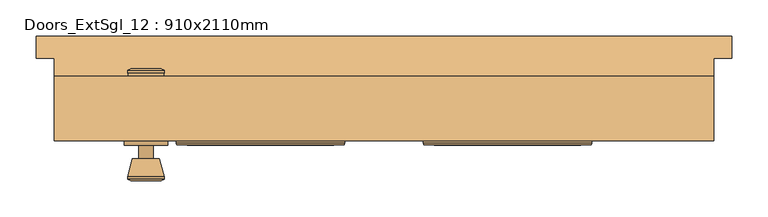
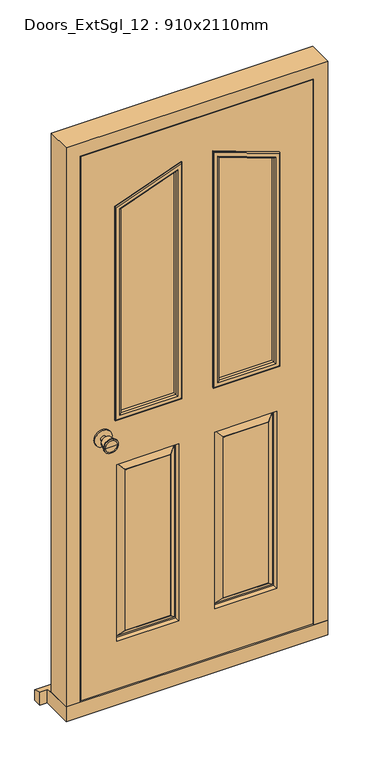
"""IFC4 building model written with IfcOpenShell, lengths in millimetres: door geometry, Doors_ExtSgl_12 : 910x2110mm."""

from ifc_helpers import new_model, si_unit, point, frame, frame_2d, origin, place, context, project, spatial, polyline, circle_curve, ellipse_curve, trimmed, segment, composite_curve, outline, extrude, faceted_brep, source, transform, mapped, element, save
from ifc_brep_helpers import plane_surface, cylinder_surface, revolved_surface, advanced_brep


def doors_extsgl_12_910x2110mm_9a09825e(model_context):
    return source(origin(), model_context, "Body", "SolidModel", [
        advanced_brep(
        [(-328.5, -18.4, 1000.0), (-318.5, -18.4, 1000.0), (-338.5, -18.4, 1000.0), (-308.0241324, -67.4, 1000.0), (-328.5, -67.4, 1000.0), (-348.9758676, -67.4, 1000.0), (-303.5, -65.5721319, 1000.0), (-353.5, -65.5721319, 1000.0), (-303.5, -62.1084537, 1000.0), (-353.5, -62.1084537, 1000.0), (-309.863764, -37.4, 1000.0), (-347.136236, -37.4, 1000.0), (-318.5, -37.4, 1000.0), (-338.5, -37.4, 1000.0)],
        [
            (0, 1),
            (1, 2, circle_curve(frame((-328.5, -18.4, 1000.0), z_axis=(0.0, 1.0, 0.0), x_axis=(-1.0, 0.0, 0.0)), 10.0)),
            (2, 0),
            (2, 1, circle_curve(frame((-328.5, -18.4, 1000.0), z_axis=(0.0, 1.0, 0.0), x_axis=(-1.0, 0.0, 0.0)), 10.0)),
            (3, 4),
            (4, 5),
            (5, 3, circle_curve(frame((-328.5, -67.4, 1000.0), z_axis=(0.0, -1.0, 0.0), x_axis=(-1.0, 0.0, 0.0)), 20.4758676)),
            (3, 5, circle_curve(frame((-328.5, -67.4, 1000.0), z_axis=(0.0, -1.0, 0.0), x_axis=(-1.0, 0.0, 0.0)), 20.4758676)),
            (6, 3),
            (5, 7),
            (7, 6, circle_curve(frame((-328.5, -65.5721319, 1000.0), z_axis=(0.0, -1.0, 0.0), x_axis=(-1.0, 0.0, 0.0)), 25.0)),
            (6, 7, circle_curve(frame((-328.5, -65.5721319, 1000.0), z_axis=(0.0, -1.0, 0.0), x_axis=(-1.0, 0.0, 0.0)), 25.0)),
            (8, 6),
            (7, 9),
            (9, 8, circle_curve(frame((-328.5, -62.1084537, 1000.0), z_axis=(0.0, -1.0, 0.0), x_axis=(-1.0, 0.0, 0.0)), 25.0)),
            (8, 9, circle_curve(frame((-328.5, -62.1084537, 1000.0), z_axis=(0.0, -1.0, 0.0), x_axis=(-1.0, 0.0, 0.0)), 25.0)),
            (10, 8),
            (9, 11),
            (11, 10, circle_curve(frame((-328.5, -37.4, 1000.0), z_axis=(0.0, -1.0, 0.0), x_axis=(-1.0, 0.0, 0.0)), 18.636236)),
            (10, 11, circle_curve(frame((-328.5, -37.4, 1000.0), z_axis=(0.0, -1.0, 0.0), x_axis=(-1.0, 0.0, 0.0)), 18.636236)),
            (12, 10),
            (11, 13),
            (13, 12, circle_curve(frame((-328.5, -37.4, 1000.0), z_axis=(0.0, -1.0, 0.0), x_axis=(-1.0, 0.0, 0.0)), 10.0)),
            (12, 13, circle_curve(frame((-328.5, -37.4, 1000.0), z_axis=(0.0, -1.0, 0.0), x_axis=(-1.0, 0.0, 0.0)), 10.0)),
            (1, 12),
            (13, 2),
        ],
        [
            plane_surface(frame((-328.5, -18.4, 1000.0), z_axis=(0.0, 1.0, 0.0), x_axis=(-1.0, 0.0, 0.0))),
            plane_surface(frame((-328.5, -67.4, 1000.0), z_axis=(0.0, -1.0, 0.0), x_axis=(-1.0, 0.0, 0.0))),
            revolved_surface(polyline([(-348.9758676, -67.4, 1000.0), (-353.5, -65.5721319, 1000.0)]), (-328.5, -18.4, 1000.0), (0.0, 1.0, 0.0)),
            cylinder_surface(frame((-328.5, -18.4, 1000.0), z_axis=(0.0, 1.0, 0.0), x_axis=(-1.0, 0.0, 0.0)), 25.0),
            revolved_surface(polyline([(-353.5, -62.1084537, 1000.0), (-347.136236, -37.4, 1000.0)]), (-328.5, -18.4, 1000.0), (0.0, 1.0, 0.0)),
            plane_surface(frame((-328.5, -37.4, 1000.0), z_axis=(0.0, 1.0, 0.0), x_axis=(-1.0, 0.0, 0.0))),
            cylinder_surface(frame((-328.5, -18.4, 1000.0), z_axis=(0.0, 1.0, 0.0), x_axis=(-1.0, 0.0, 0.0)), 10.0),
        ],
        [
            (0, [[1, 2, 3]]),
            (0, [[-3, 4, -1]]),
            (1, [[5, 6, 7]]),
            (1, [[-6, -5, 8]]),
            (2, [[9, -7, 10, 11]]),
            (2, [[-10, -8, -9, 12]]),
            (3, [[13, -11, 14, 15]]),
            (3, [[-14, -12, -13, 16]]),
            (4, [[17, -15, 18, 19]]),
            (4, [[-18, -16, -17, 20]]),
            (5, [[21, -19, 22, 23]]),
            (5, [[-22, -20, -21, 24]]),
            (6, [[25, -23, 26, -2]]),
            (6, [[-26, -24, -25, -4]]),
        ],
    ),
        extrude(outline(composite_curve([segment(trimmed(circle_curve(frame_2d((1000.0, -328.5)), 30.0), [point((1000.0, -358.5))], [point((1000.0, -298.5))], False, "CARTESIAN"), True, "CONTINUOUS"), segment(trimmed(circle_curve(frame_2d((1000.0, -328.5)), 30.0), [point((1000.0, -298.5))], [point((1000.0, -358.5))], False, "CARTESIAN"), True, "CONTINUOUS")], self_intersect=False)), frame((0.0, -18.4, 0.0), z_axis=(0.0, 1.0, 0.0), x_axis=(0.0, 0.0, 1.0)), (0.0, 0.0, 1.0), 6.0),
        advanced_brep(
        [(-328.5, 37.6, 1000.0), (-338.5, 37.6, 1000.0), (-318.5, 37.6, 1000.0), (-308.0241324, 86.6, 1000.0), (-348.9758676, 86.6, 1000.0), (-328.5, 86.6, 1000.0), (-303.5, 84.7721319, 1000.0), (-353.5, 84.7721319, 1000.0), (-303.5, 81.3084537, 1000.0), (-353.5, 81.3084537, 1000.0), (-309.863764, 56.6, 1000.0), (-347.136236, 56.6, 1000.0), (-318.5, 56.6, 1000.0), (-338.5, 56.6, 1000.0)],
        [
            (0, 1),
            (1, 2, circle_curve(frame((-328.5, 37.6, 1000.0), z_axis=(0.0, -1.0, 0.0), x_axis=(-1.0, 0.0, 0.0)), 10.0)),
            (2, 0),
            (2, 1, circle_curve(frame((-328.5, 37.6, 1000.0), z_axis=(0.0, -1.0, 0.0), x_axis=(-1.0, 0.0, 0.0)), 10.0)),
            (3, 4, circle_curve(frame((-328.5, 86.6, 1000.0), z_axis=(0.0, 1.0, 0.0), x_axis=(-1.0, 0.0, 0.0)), 20.4758676)),
            (4, 5),
            (5, 3),
            (4, 3, circle_curve(frame((-328.5, 86.6, 1000.0), z_axis=(0.0, 1.0, 0.0), x_axis=(-1.0, 0.0, 0.0)), 20.4758676)),
            (6, 7, circle_curve(frame((-328.5, 84.7721319, 1000.0), z_axis=(0.0, 1.0, 0.0), x_axis=(-1.0, 0.0, 0.0)), 25.0)),
            (7, 4),
            (3, 6),
            (7, 6, circle_curve(frame((-328.5, 84.7721319, 1000.0), z_axis=(0.0, 1.0, 0.0), x_axis=(-1.0, 0.0, 0.0)), 25.0)),
            (8, 9, circle_curve(frame((-328.5, 81.3084537, 1000.0), z_axis=(0.0, 1.0, 0.0), x_axis=(-1.0, 0.0, 0.0)), 25.0)),
            (9, 7),
            (6, 8),
            (9, 8, circle_curve(frame((-328.5, 81.3084537, 1000.0), z_axis=(0.0, 1.0, 0.0), x_axis=(-1.0, 0.0, 0.0)), 25.0)),
            (10, 11, circle_curve(frame((-328.5, 56.6, 1000.0), z_axis=(0.0, 1.0, 0.0), x_axis=(-1.0, 0.0, 0.0)), 18.636236)),
            (11, 9),
            (8, 10),
            (11, 10, circle_curve(frame((-328.5, 56.6, 1000.0), z_axis=(0.0, 1.0, 0.0), x_axis=(-1.0, 0.0, 0.0)), 18.636236)),
            (12, 13, circle_curve(frame((-328.5, 56.6, 1000.0), z_axis=(0.0, 1.0, 0.0), x_axis=(-1.0, 0.0, 0.0)), 10.0)),
            (13, 11),
            (10, 12),
            (13, 12, circle_curve(frame((-328.5, 56.6, 1000.0), z_axis=(0.0, 1.0, 0.0), x_axis=(-1.0, 0.0, 0.0)), 10.0)),
            (1, 13),
            (12, 2),
        ],
        [
            plane_surface(frame((-328.5, 37.6, 1000.0), z_axis=(0.0, -1.0, 0.0), x_axis=(-1.0, 0.0, 0.0))),
            plane_surface(frame((-328.5, 86.6, 1000.0), z_axis=(0.0, 1.0, 0.0), x_axis=(-1.0, 0.0, 0.0))),
            revolved_surface(polyline([(-348.9758676, 86.6, 1000.0), (-353.5, 84.7721319, 1000.0)]), (-328.5, 37.6, 1000.0), (0.0, -1.0, 0.0)),
            cylinder_surface(frame((-328.5, 37.6, 1000.0), z_axis=(0.0, -1.0, 0.0), x_axis=(-1.0, 0.0, 0.0)), 25.0),
            revolved_surface(polyline([(-353.5, 81.3084537, 1000.0), (-347.136236, 56.6, 1000.0)]), (-328.5, 37.6, 1000.0), (0.0, -1.0, 0.0)),
            plane_surface(frame((-328.5, 56.6, 1000.0), z_axis=(0.0, -1.0, 0.0), x_axis=(-1.0, 0.0, 0.0))),
            cylinder_surface(frame((-328.5, 37.6, 1000.0), z_axis=(0.0, -1.0, 0.0), x_axis=(-1.0, 0.0, 0.0)), 10.0),
        ],
        [
            (0, [[1, 2, 3]]),
            (0, [[-3, 4, -1]]),
            (1, [[5, 6, 7]]),
            (1, [[8, -7, -6]]),
            (2, [[9, 10, -5, 11]]),
            (2, [[12, -11, -8, -10]]),
            (3, [[13, 14, -9, 15]]),
            (3, [[16, -15, -12, -14]]),
            (4, [[17, 18, -13, 19]]),
            (4, [[20, -19, -16, -18]]),
            (5, [[21, 22, -17, 23]]),
            (5, [[24, -23, -20, -22]]),
            (6, [[-2, 25, -21, 26]]),
            (6, [[-4, -26, -24, -25]]),
        ],
    ),
        extrude(outline(composite_curve([segment(trimmed(circle_curve(frame_2d((1000.0, -328.5)), 30.0), [point((1000.0, -358.5))], [point((1000.0, -298.5))], False, "CARTESIAN"), True, "CONTINUOUS"), segment(trimmed(circle_curve(frame_2d((1000.0, -328.5)), 30.0), [point((1000.0, -298.5))], [point((1000.0, -358.5))], False, "CARTESIAN"), True, "CONTINUOUS")], self_intersect=False)), frame((0.0, 31.6, 0.0), z_axis=(0.0, 1.0, 0.0), x_axis=(0.0, 0.0, 1.0)), (0.0, 0.0, 1.0), 6.0),
        faceted_brep([(384.5, 76.6, 54.5), (455.0, 76.6, 54.5), (455.0, -12.4, 54.5), (406.5, -12.4, 54.5), (406.5, 34.6, 54.5), (384.5, 34.6, 54.5), (384.5, 76.6, 2039.5), (-384.5, 76.6, 2039.5), (-384.5, 76.6, 54.5), (-455.0, 76.6, 54.5), (-455.0, 76.6, 2110.0), (455.0, 76.6, 2110.0), (455.0, -12.4, 2110.0), (-455.0, -12.4, 2110.0), (-455.0, -12.4, 54.5), (-406.5, -12.4, 54.5), (-406.5, -12.4, 2061.5), (406.5, -12.4, 2061.5), (406.5, 34.6, 2061.5), (-406.5, 34.6, 2061.5), (-406.5, 34.6, 54.5), (-384.5, 34.6, 54.5), (-384.5, 34.6, 2039.5), (384.5, 34.6, 2039.5)], [[[0, 1, 2, 3, 4, 5]], [[1, 0, 6, 7, 8, 9, 10, 11]], [[2, 1, 11, 12]], [[3, 2, 12, 13, 14, 15, 16, 17]], [[4, 3, 17, 18]], [[5, 4, 18, 19, 20, 21, 22, 23]], [[0, 5, 23, 6]], [[8, 7, 22, 21]], [[9, 8, 21, 20, 15, 14]], [[10, 9, 14, 13]], [[16, 15, 20, 19]], [[11, 10, 13, 12]], [[17, 16, 19, 18]], [[7, 6, 23, 22]]]),
        faceted_brep([(403.5, -12.4, 58.5), (403.5, -12.4, 2058.5), (-404.4250294, -12.4, 2058.5), (-404.4250294, -12.4, 58.5), (62.5, -12.4, 1058.5), (62.5, -12.4, 1908.5), (278.5, -12.4, 1829.8824294), (278.5, -12.4, 1058.5), (-278.5, -12.4, 1058.5), (-278.5, -12.4, 1829.8824294), (-62.5, -12.4, 1908.5), (-62.5, -12.4, 1058.5), (-62.5, -12.4, 883.5), (-62.5, -12.4, 233.5), (-278.5, -12.4, 233.5), (-278.5, -12.4, 883.5), (278.5, -12.4, 883.5), (278.5, -12.4, 233.5), (62.5, -12.4, 233.5), (62.5, -12.4, 883.5), (-92.5, -12.4, 263.5), (-92.5, -12.4, 853.5), (-248.5, -12.4, 853.5), (-248.5, -12.4, 263.5), (248.5, -12.4, 263.5), (248.5, -12.4, 853.5), (92.5, -12.4, 853.5), (92.5, -12.4, 263.5), (403.5, 31.6, 58.5), (-404.4250294, 31.6, 58.5), (-404.4250294, 31.6, 2058.5), (403.5, 31.6, 2058.5), (62.5, 31.6, 1058.5), (278.5, 31.6, 1058.5), (278.5, 31.6, 1829.8824294), (62.5, 31.6, 1908.5), (-278.5, 31.6, 1058.5), (-62.5, 31.6, 1058.5), (-62.5, 31.6, 1908.5), (-278.5, 31.6, 1829.8824294), (62.5, 31.6, 883.5), (62.5, 31.6, 233.5), (278.5, 31.6, 233.5), (278.5, 31.6, 883.5), (-278.5, 31.6, 883.5), (-278.5, 31.6, 233.5), (-62.5, 31.6, 233.5), (-62.5, 31.6, 883.5), (92.5, 31.6, 263.5), (92.5, 31.6, 853.5), (248.5, 31.6, 853.5), (248.5, 31.6, 263.5), (-248.5, 31.6, 263.5), (-248.5, 31.6, 853.5), (-92.5, 31.6, 853.5), (-92.5, 31.6, 263.5), (65.5, 16.6, 880.5), (65.5, 16.6, 236.5), (90.5, 30.6, 855.5), (90.5, 30.6, 261.5), (70.5, 16.6, 241.5), (70.5, 16.6, 875.5), (92.5, 30.6, 263.5), (92.5, 30.6, 853.5), (275.5, 16.6, 236.5), (250.5, 30.6, 261.5), (270.5, 16.6, 241.5), (248.5, 30.6, 263.5), (275.5, 16.6, 880.5), (250.5, 30.6, 855.5), (270.5, 16.6, 875.5), (248.5, 30.6, 853.5), (-275.5, 16.6, 880.5), (-275.5, 16.6, 236.5), (-250.5, 30.6, 855.5), (-250.5, 30.6, 261.5), (-270.5, 16.6, 241.5), (-270.5, 16.6, 875.5), (-248.5, 30.6, 263.5), (-248.5, 30.6, 853.5), (-65.5, 16.6, 236.5), (-90.5, 30.6, 261.5), (-70.5, 16.6, 241.5), (-92.5, 30.6, 263.5), (-65.5, 16.6, 880.5), (-90.5, 30.6, 855.5), (-70.5, 16.6, 875.5), (-92.5, 30.6, 853.5), (-92.5, -11.4, 263.5), (-92.5, -11.4, 853.5), (-70.5, 2.6, 241.5), (-70.5, 2.6, 875.5), (-90.5, -11.4, 855.5), (-90.5, -11.4, 261.5), (-65.5, 2.6, 880.5), (-65.5, 2.6, 236.5), (-248.5, -11.4, 853.5), (-270.5, 2.6, 875.5), (-250.5, -11.4, 855.5), (-275.5, 2.6, 880.5), (-248.5, -11.4, 263.5), (-270.5, 2.6, 241.5), (-250.5, -11.4, 261.5), (-275.5, 2.6, 236.5), (275.5, 2.6, 880.5), (275.5, 2.6, 236.5), (250.5, -11.4, 855.5), (250.5, -11.4, 261.5), (270.5, 2.6, 241.5), (270.5, 2.6, 875.5), (248.5, -11.4, 263.5), (248.5, -11.4, 853.5), (65.5, 2.6, 236.5), (90.5, -11.4, 261.5), (70.5, 2.6, 241.5), (92.5, -11.4, 263.5), (65.5, 2.6, 880.5), (90.5, -11.4, 855.5), (70.5, 2.6, 875.5), (92.5, -11.4, 853.5)], [[[0, 1, 2, 3], [4, 5, 6, 7], [8, 9, 10, 11], [12, 13, 14, 15], [16, 17, 18, 19]], [[20, 21, 22, 23]], [[24, 25, 26, 27]], [[28, 29, 30, 31], [32, 33, 34, 35], [36, 37, 38, 39], [40, 41, 42, 43], [44, 45, 46, 47]], [[48, 49, 50, 51]], [[52, 53, 54, 55]], [[1, 0, 28, 31]], [[2, 1, 31, 30]], [[3, 2, 30, 29]], [[0, 3, 29, 28]], [[5, 4, 32, 35]], [[6, 5, 35, 34]], [[7, 6, 34, 33]], [[4, 7, 33, 32]], [[9, 8, 36, 39]], [[10, 9, 39, 38]], [[11, 10, 38, 37]], [[8, 11, 37, 36]], [[56, 57, 41, 40]], [[58, 59, 60, 61]], [[48, 62, 63, 49]], [[41, 57, 64, 42]], [[60, 59, 65, 66]], [[62, 48, 51, 67]], [[42, 64, 68, 43]], [[66, 65, 69, 70]], [[67, 51, 50, 71]], [[56, 40, 43, 68]], [[57, 56, 68, 64], [61, 60, 66, 70]], [[58, 61, 70, 69]], [[59, 58, 69, 65], [63, 62, 67, 71]], [[49, 63, 71, 50]], [[72, 73, 45, 44]], [[74, 75, 76, 77]], [[52, 78, 79, 53]], [[45, 73, 80, 46]], [[76, 75, 81, 82]], [[78, 52, 55, 83]], [[46, 80, 84, 47]], [[82, 81, 85, 86]], [[83, 55, 54, 87]], [[72, 44, 47, 84]], [[73, 72, 84, 80], [77, 76, 82, 86]], [[74, 77, 86, 85]], [[75, 74, 85, 81], [79, 78, 83, 87]], [[53, 79, 87, 54]], [[88, 89, 21, 20]], [[90, 91, 92, 93]], [[12, 94, 95, 13]], [[21, 89, 96, 22]], [[92, 91, 97, 98]], [[94, 12, 15, 99]], [[22, 96, 100, 23]], [[98, 97, 101, 102]], [[99, 15, 14, 103]], [[88, 20, 23, 100]], [[93, 92, 98, 102], [89, 88, 100, 96]], [[90, 93, 102, 101]], [[95, 94, 99, 103], [91, 90, 101, 97]], [[13, 95, 103, 14]], [[104, 105, 17, 16]], [[106, 107, 108, 109]], [[24, 110, 111, 25]], [[17, 105, 112, 18]], [[108, 107, 113, 114]], [[110, 24, 27, 115]], [[18, 112, 116, 19]], [[114, 113, 117, 118]], [[115, 27, 26, 119]], [[104, 16, 19, 116]], [[105, 104, 116, 112], [109, 108, 114, 118]], [[106, 109, 118, 117]], [[107, 106, 117, 113], [111, 110, 115, 119]], [[25, 111, 119, 26]]]),
        faceted_brep([(480.0, 131.6, 0.0), (480.0, 131.6, 38.5947221), (480.0, 101.6, 47.2703282), (480.0, 101.6, 0.0), (-480.0, 131.6, 38.5947221), (-480.0, 131.6, 0.0), (-480.0, 101.6, 0.0), (-480.0, 101.6, 47.2703282), (455.0, 101.6, 0.0), (455.0, -12.4, 0.0), (-455.0, -12.4, 0.0), (-455.0, 101.6, 0.0), (-455.0, 101.6, 47.2703282), (-455.0, 76.6, 54.5), (455.0, 76.6, 54.5), (455.0, 101.6, 47.2703282), (-455.0, -12.4, 54.5), (455.0, -12.4, 54.5)], [[[0, 1, 2, 3]], [[4, 5, 6, 7]], [[5, 0, 3, 8, 9, 10, 11, 6]], [[1, 0, 5, 4]], [[1, 4, 7, 12, 13, 14, 15, 2]], [[13, 16, 17, 14]], [[16, 10, 9, 17]], [[12, 11, 10, 16, 13]], [[11, 12, 7, 6]], [[8, 15, 14, 17, 9]], [[15, 8, 3, 2]]]),
        extrude(outline(polyline([(1058.5, 278.5), (1829.8824294, 278.5), (1908.5, 62.5), (1058.5, 62.5), (1058.5, 278.5)])), frame((0.0, -2.4, 0.0), z_axis=(0.0, 1.0, 0.0), x_axis=(0.0, 0.0, 1.0)), (0.0, 0.0, 1.0), 24.0),
        extrude(outline(polyline([(1058.5, -62.5), (1908.5, -62.5), (1829.8824294, -278.5), (1058.5, -278.5), (1058.5, -62.5)])), frame((0.0, -2.4, 0.0), z_axis=(0.0, 1.0, 0.0), x_axis=(0.0, 0.0, 1.0)), (0.0, 0.0, 1.0), 24.0),
        advanced_brep(
        [(286.5, 35.6, 1835.4840897), (286.5, 31.6, 1835.4840897), (286.5, 31.6, 1050.5), (286.5, 35.6, 1050.5), (284.5, 37.6, 1834.0836746), (284.5, 37.6, 1052.5), (266.5, 32.6, 1821.4799389), (271.5, 37.6, 1824.9809766), (271.5, 37.6, 1065.5), (266.5, 32.6, 1070.5), (266.5, 21.6, 1821.4799389), (266.5, 21.6, 1070.5), (278.5, 31.6, 1829.8824294), (278.5, 21.6, 1829.8824294), (278.5, 21.6, 1058.5), (278.5, 31.6, 1058.5), (54.5, 31.6, 1050.5), (54.5, 35.6, 1050.5), (56.5, 37.6, 1052.5), (69.5, 37.6, 1065.5), (74.5, 32.6, 1070.5), (74.5, 21.6, 1070.5), (62.5, 21.6, 1058.5), (62.5, 31.6, 1058.5), (54.5, 31.6, 1919.9251841), (54.5, 35.6, 1919.9251841), (56.5, 37.6, 1917.068888), (69.5, 37.6, 1898.502964), (74.5, 32.6, 1891.3622239), (74.5, 21.6, 1891.3622239), (62.5, 21.6, 1908.5), (62.5, 31.6, 1908.5)],
        [
            (0, 1),
            (1, 2),
            (2, 3),
            (3, 0),
            (4, 0, ellipse_curve(frame((284.5, 35.6, 1834.0836746), z_axis=(0.5735764363510463, 0.0, -0.8191520442889918), x_axis=(0.8191520442889918, 0.0, 0.5735764363510459)), 2.4415492, 2.0)),
            (3, 5, ellipse_curve(frame((284.5, 35.6, 1052.5), z_axis=(0.7071067811865475, 0.0, 0.7071067811865475), x_axis=(-0.7071067811865474, 0.0, 0.7071067811865476)), 2.8284271, 2.0)),
            (5, 4),
            (6, 7, ellipse_curve(frame((271.5, 32.6, 1824.9809766), z_axis=(0.5735764363510463, 0.0, -0.8191520442889918), x_axis=(0.8191520442889918, 0.0, 0.5735764363510459)), 6.1038729, 5.0)),
            (7, 8),
            (8, 9, ellipse_curve(frame((271.5, 32.6, 1065.5), z_axis=(0.7071067811865475, 0.0, 0.7071067811865475), x_axis=(-0.7071067811865474, 0.0, 0.7071067811865476)), 7.0710678, 5.0)),
            (9, 6),
            (10, 6),
            (9, 11),
            (11, 10),
            (12, 13),
            (13, 14),
            (14, 15),
            (15, 12),
            (2, 16),
            (16, 17),
            (17, 3),
            (17, 18, ellipse_curve(frame((56.5, 35.6, 1052.5), z_axis=(0.7071067811865475, 0.0, -0.7071067811865475), x_axis=(0.7071067811865476, 0.0, 0.7071067811865474)), 2.8284271, 2.0)),
            (18, 5),
            (8, 19),
            (19, 20, ellipse_curve(frame((69.5, 32.6, 1065.5), z_axis=(0.7071067811865475, 0.0, -0.7071067811865475), x_axis=(0.7071067811865476, 0.0, 0.7071067811865474)), 7.0710678, 5.0)),
            (20, 9),
            (20, 21),
            (21, 11),
            (14, 22),
            (22, 23),
            (23, 15),
            (16, 24),
            (24, 25),
            (25, 17),
            (25, 26, ellipse_curve(frame((56.5, 35.6, 1917.068888), z_axis=(-0.8191520442889917, 0.0, -0.5735764363510462), x_axis=(0.5735764363510462, 0.0, -0.8191520442889918)), 3.4868936, 2.0)),
            (26, 18),
            (19, 27),
            (27, 28, ellipse_curve(frame((69.5, 32.6, 1898.502964), z_axis=(-0.8191520442889917, 0.0, -0.5735764363510462), x_axis=(0.5735764363510462, 0.0, -0.8191520442889918)), 8.717234, 5.0)),
            (28, 20),
            (28, 29),
            (29, 21),
            (22, 30),
            (30, 31),
            (31, 23),
            (24, 1),
            (0, 25),
            (4, 26),
            (7, 27),
            (6, 28),
            (10, 29),
            (13, 30),
            (12, 31),
        ],
        [
            plane_surface(frame((286.5, 31.6, 1835.4840897), z_axis=(1.0, 0.0, 0.0), x_axis=(0.0, 0.0, -1.0))),
            cylinder_surface(frame((284.5, 35.6, 1829.8824294), z_axis=(0.0, 0.0, 1.0), x_axis=(1.0, 0.0, 0.0)), 2.0),
            cylinder_surface(frame((271.5, 32.6, 1829.8824294), z_axis=(0.0, 0.0, 1.0), x_axis=(1.0, 0.0, 0.0)), 5.0),
            plane_surface(frame((266.5, 32.6, 1821.4799389), z_axis=(-1.0, 0.0, 0.0), x_axis=(0.0, 0.0, -1.0))),
            plane_surface(frame((278.5, 21.6, 1829.8824294), z_axis=(1.0, 0.0, 0.0), x_axis=(0.0, 0.0, -1.0))),
            plane_surface(frame((286.5, 31.6, 1050.5), z_axis=(0.0, 0.0, -1.0), x_axis=(-1.0, 0.0, 0.0))),
            cylinder_surface(frame((278.5, 35.6, 1052.5), z_axis=(1.0, 0.0, 0.0), x_axis=(0.0, 0.0, -1.0)), 2.0),
            cylinder_surface(frame((278.5, 32.6, 1065.5), z_axis=(1.0, 0.0, 0.0), x_axis=(0.0, 0.0, -1.0)), 5.0),
            plane_surface(frame((266.5, 32.6, 1070.5), z_axis=(0.0, 0.0, 1.0), x_axis=(-1.0, 0.0, 0.0))),
            plane_surface(frame((278.5, 21.6, 1058.5), z_axis=(0.0, 0.0, -1.0), x_axis=(-1.0, 0.0, 0.0))),
            plane_surface(frame((54.5, 31.6, 1050.5), z_axis=(-1.0, 0.0, 0.0), x_axis=(0.0, 0.0, 1.0))),
            cylinder_surface(frame((56.5, 35.6, 1058.5), z_axis=(0.0, 0.0, -1.0), x_axis=(-1.0, 0.0, 0.0)), 2.0),
            cylinder_surface(frame((69.5, 32.6, 1058.5), z_axis=(0.0, 0.0, -1.0), x_axis=(-1.0, 0.0, 0.0)), 5.0),
            plane_surface(frame((74.5, 32.6, 1070.5), z_axis=(1.0, 0.0, 0.0), x_axis=(0.0, 0.0, 1.0))),
            plane_surface(frame((62.5, 21.6, 1058.5), z_axis=(-1.0, 0.0, 0.0), x_axis=(0.0, 0.0, 1.0))),
            plane_surface(frame((54.5, 31.6, 1919.9251841), z_axis=(0.3420201433256683, 0.0, 0.9396926207859085), x_axis=(0.9396926207859085, 0.0, -0.3420201433256683))),
            cylinder_surface(frame((64.5521209, 35.6, 1914.1381557), z_axis=(-0.9396926207859085, 0.0, 0.34202014332566844), x_axis=(0.34202014332566844, 0.0, 0.9396926207859085)), 2.0),
            plane_surface(frame((56.5, 37.6, 1917.068888), z_axis=(0.0, 1.0, 0.0), x_axis=(0.9396926207859085, 0.0, -0.34202014332566844))),
            cylinder_surface(frame((60.105859, 32.6, 1901.9221517), z_axis=(-0.9396926207859085, 0.0, 0.34202014332566844), x_axis=(0.34202014332566844, 0.0, 0.9396926207859085)), 5.0),
            plane_surface(frame((74.5, 32.6, 1891.3622239), z_axis=(-0.34202014332566844, 0.0, -0.9396926207859085), x_axis=(0.9396926207859085, 0.0, -0.34202014332566844))),
            plane_surface(frame((74.5, 21.6, 1891.3622239), z_axis=(0.0, -1.0, 0.0), x_axis=(0.9396926207859088, 0.0, -0.3420201433256677))),
            plane_surface(frame((62.5, 21.6, 1908.5), z_axis=(0.34202014332566905, 0.0, 0.9396926207859083), x_axis=(0.9396926207859083, 0.0, -0.34202014332566905))),
            plane_surface(frame((62.5, 31.6, 1908.5), z_axis=(0.0, -1.0, 0.0), x_axis=(0.9396926207859083, 0.0, -0.3420201433256691))),
        ],
        [
            (0, [[1, 2, 3, 4]]),
            (1, [[5, -4, 6, 7]]),
            (2, [[8, 9, 10, 11]]),
            (3, [[12, -11, 13, 14]]),
            (4, [[15, 16, 17, 18]]),
            (5, [[-3, 19, 20, 21]]),
            (6, [[-6, -21, 22, 23]]),
            (7, [[-10, 24, 25, 26]]),
            (8, [[-13, -26, 27, 28]]),
            (9, [[-17, 29, 30, 31]]),
            (10, [[-20, 32, 33, 34]]),
            (11, [[-22, -34, 35, 36]]),
            (12, [[-25, 37, 38, 39]]),
            (13, [[-27, -39, 40, 41]]),
            (14, [[-30, 42, 43, 44]]),
            (15, [[-33, 45, -1, 46]]),
            (16, [[-35, -46, -5, 47]]),
            (17, [[-23, -36, -47, -7], [48, -37, -24, -9]]),
            (18, [[-38, -48, -8, 49]]),
            (19, [[-40, -49, -12, 50]]),
            (20, [[51, -42, -29, -16], [-28, -41, -50, -14]]),
            (21, [[-43, -51, -15, 52]]),
            (22, [[-45, -32, -19, -2], [-31, -44, -52, -18]]),
        ],
    ),
        advanced_brep(
        [(-54.5, 35.6, 1050.5), (-54.5, 31.6, 1050.5), (-286.5, 31.6, 1050.5), (-286.5, 35.6, 1050.5), (-56.5, 37.6, 1052.5), (-284.5, 37.6, 1052.5), (-74.5, 32.6, 1070.5), (-69.5, 37.6, 1065.5), (-271.5, 37.6, 1065.5), (-266.5, 32.6, 1070.5), (-74.5, 21.6, 1070.5), (-266.5, 21.6, 1070.5), (-62.5, 31.6, 1058.5), (-62.5, 21.6, 1058.5), (-278.5, 21.6, 1058.5), (-278.5, 31.6, 1058.5), (-286.5, 31.6, 1835.4840897), (-286.5, 35.6, 1835.4840897), (-284.5, 37.6, 1834.0836746), (-271.5, 37.6, 1824.9809766), (-266.5, 32.6, 1821.4799389), (-266.5, 21.6, 1821.4799389), (-278.5, 21.6, 1829.8824294), (-278.5, 31.6, 1829.8824294), (-54.5, 31.6, 1919.9251841), (-54.5, 35.6, 1919.9251841), (-56.5, 37.6, 1917.068888), (-69.5, 37.6, 1898.502964), (-74.5, 32.6, 1891.3622239), (-74.5, 21.6, 1891.3622239), (-62.5, 21.6, 1908.5), (-62.5, 31.6, 1908.5)],
        [
            (0, 1),
            (1, 2),
            (2, 3),
            (3, 0),
            (4, 0, ellipse_curve(frame((-56.5, 35.6, 1052.5), z_axis=(-0.7071067811865475, 0.0, -0.7071067811865475), x_axis=(0.7071067811865476, 0.0, -0.7071067811865475)), 2.8284271, 2.0)),
            (3, 5, ellipse_curve(frame((-284.5, 35.6, 1052.5), z_axis=(0.7071067811865476, 0.0, -0.7071067811865475), x_axis=(0.7071067811865475, 0.0, 0.7071067811865475)), 2.8284271, 2.0)),
            (5, 4),
            (6, 7, ellipse_curve(frame((-69.5, 32.6, 1065.5), z_axis=(-0.7071067811865475, 0.0, -0.7071067811865475), x_axis=(0.7071067811865476, 0.0, -0.7071067811865475)), 7.0710678, 5.0)),
            (7, 8),
            (8, 9, ellipse_curve(frame((-271.5, 32.6, 1065.5), z_axis=(0.7071067811865476, 0.0, -0.7071067811865475), x_axis=(0.7071067811865475, 0.0, 0.7071067811865475)), 7.0710678, 5.0)),
            (9, 6),
            (10, 6),
            (9, 11),
            (11, 10),
            (12, 13),
            (13, 14),
            (14, 15),
            (15, 12),
            (2, 16),
            (16, 17),
            (17, 3),
            (17, 18, ellipse_curve(frame((-284.5, 35.6, 1834.0836746), z_axis=(-0.5735764363510245, 0.0, -0.8191520442890069), x_axis=(0.8191520442890068, 0.0, -0.5735764363510246)), 2.4415492, 2.0)),
            (18, 5),
            (8, 19),
            (19, 20, ellipse_curve(frame((-271.5, 32.6, 1824.9809766), z_axis=(-0.5735764363510245, 0.0, -0.8191520442890069), x_axis=(0.8191520442890068, 0.0, -0.5735764363510246)), 6.1038729, 5.0)),
            (20, 9),
            (20, 21),
            (21, 11),
            (14, 22),
            (22, 23),
            (23, 15),
            (16, 24),
            (24, 25),
            (25, 17),
            (25, 26, ellipse_curve(frame((-56.5, 35.6, 1917.068888), z_axis=(-0.8191520442890069, 0.0, 0.5735764363510246), x_axis=(-0.5735764363510246, 0.0, -0.8191520442890069)), 3.4868936, 2.0)),
            (26, 18),
            (19, 27),
            (27, 28, ellipse_curve(frame((-69.5, 32.6, 1898.502964), z_axis=(-0.8191520442890069, 0.0, 0.5735764363510246), x_axis=(-0.5735764363510246, 0.0, -0.8191520442890069)), 8.717234, 5.0)),
            (28, 20),
            (28, 29),
            (29, 21),
            (22, 30),
            (30, 31),
            (31, 23),
            (24, 1),
            (0, 25),
            (4, 26),
            (7, 27),
            (6, 28),
            (10, 29),
            (13, 30),
            (12, 31),
        ],
        [
            plane_surface(frame((-54.5, 31.6, 1050.5), z_axis=(0.0, 0.0, -1.0), x_axis=(-1.0, 0.0, 0.0))),
            cylinder_surface(frame((-62.5, 35.6, 1052.5), z_axis=(1.0, 0.0, 0.0), x_axis=(0.0, 0.0, -1.0)), 2.0),
            cylinder_surface(frame((-62.5, 32.6, 1065.5), z_axis=(1.0, 0.0, 0.0), x_axis=(0.0, 0.0, -1.0)), 5.0),
            plane_surface(frame((-74.5, 32.6, 1070.5), z_axis=(0.0, 0.0, 1.0), x_axis=(-1.0, 0.0, 0.0))),
            plane_surface(frame((-62.5, 21.6, 1058.5), z_axis=(0.0, 0.0, -1.0), x_axis=(-1.0, 0.0, 0.0))),
            plane_surface(frame((-286.5, 31.6, 1050.5), z_axis=(-1.0, 0.0, 0.0), x_axis=(0.0, 0.0, 1.0))),
            cylinder_surface(frame((-284.5, 35.6, 1058.5), z_axis=(0.0, 0.0, -1.0), x_axis=(-1.0, 0.0, 0.0)), 2.0),
            cylinder_surface(frame((-271.5, 32.6, 1058.5), z_axis=(0.0, 0.0, -1.0), x_axis=(-1.0, 0.0, 0.0)), 5.0),
            plane_surface(frame((-266.5, 32.6, 1070.5), z_axis=(1.0, 0.0, 0.0), x_axis=(0.0, 0.0, 1.0))),
            plane_surface(frame((-278.5, 21.6, 1058.5), z_axis=(-1.0, 0.0, 0.0), x_axis=(0.0, 0.0, 1.0))),
            plane_surface(frame((-286.5, 31.6, 1835.4840897), z_axis=(-0.34202014332571895, 0.0, 0.9396926207858901), x_axis=(0.9396926207858901, 0.0, 0.34202014332571895))),
            cylinder_surface(frame((-280.5521209, 35.6, 1835.5205851), z_axis=(-0.9396926207858904, 0.0, -0.3420201433257182), x_axis=(-0.3420201433257182, 0.0, 0.9396926207858904)), 2.0),
            cylinder_surface(frame((-276.105859, 32.6, 1823.3045811), z_axis=(-0.9396926207858904, 0.0, -0.3420201433257182), x_axis=(-0.3420201433257182, 0.0, 0.9396926207858904)), 5.0),
            plane_surface(frame((-266.5, 32.6, 1821.4799389), z_axis=(0.3420201433257189, 0.0, -0.9396926207858901), x_axis=(0.9396926207858901, 0.0, 0.3420201433257189))),
            plane_surface(frame((-278.5, 21.6, 1829.8824294), z_axis=(-0.3420201433257181, 0.0, 0.9396926207858906), x_axis=(0.9396926207858906, 0.0, 0.3420201433257181))),
            plane_surface(frame((-54.5, 31.6, 1919.9251841), z_axis=(1.0, 0.0, 0.0), x_axis=(0.0, 0.0, -1.0))),
            cylinder_surface(frame((-56.5, 35.6, 1908.5), z_axis=(0.0, 0.0, 1.0), x_axis=(1.0, 0.0, 0.0)), 2.0),
            plane_surface(frame((-56.5, 37.6, 1917.068888), z_axis=(0.0, 1.0, 0.0), x_axis=(0.0, 0.0, -1.0))),
            cylinder_surface(frame((-69.5, 32.6, 1908.5), z_axis=(0.0, 0.0, 1.0), x_axis=(1.0, 0.0, 0.0)), 5.0),
            plane_surface(frame((-74.5, 32.6, 1891.3622239), z_axis=(-1.0, 0.0, 0.0), x_axis=(0.0, 0.0, -1.0))),
            plane_surface(frame((-74.5, 21.6, 1891.3622239), z_axis=(0.0, -1.0, 0.0), x_axis=(0.0, 0.0, -1.0))),
            plane_surface(frame((-62.5, 21.6, 1908.5), z_axis=(1.0, 0.0, 0.0), x_axis=(0.0, 0.0, -1.0))),
            plane_surface(frame((-62.5, 31.6, 1908.5), z_axis=(0.0, -1.0, 0.0), x_axis=(0.0, 0.0, -1.0))),
        ],
        [
            (0, [[1, 2, 3, 4]]),
            (1, [[5, -4, 6, 7]]),
            (2, [[8, 9, 10, 11]]),
            (3, [[12, -11, 13, 14]]),
            (4, [[15, 16, 17, 18]]),
            (5, [[-3, 19, 20, 21]]),
            (6, [[-6, -21, 22, 23]]),
            (7, [[-10, 24, 25, 26]]),
            (8, [[-13, -26, 27, 28]]),
            (9, [[-17, 29, 30, 31]]),
            (10, [[-20, 32, 33, 34]]),
            (11, [[-22, -34, 35, 36]]),
            (12, [[-25, 37, 38, 39]]),
            (13, [[-27, -39, 40, 41]]),
            (14, [[-30, 42, 43, 44]]),
            (15, [[-33, 45, -1, 46]]),
            (16, [[-35, -46, -5, 47]]),
            (17, [[-23, -36, -47, -7], [48, -37, -24, -9]]),
            (18, [[-38, -48, -8, 49]]),
            (19, [[-40, -49, -12, 50]]),
            (20, [[51, -42, -29, -16], [-28, -41, -50, -14]]),
            (21, [[-43, -51, -15, 52]]),
            (22, [[-45, -32, -19, -2], [-31, -44, -52, -18]]),
        ],
    ),
        advanced_brep(
        [(-278.5, -2.4, 1829.8824294), (-278.5, -12.4, 1829.8824294), (-62.5, -12.4, 1908.5), (-62.5, -2.4, 1908.5), (-266.5, -13.4, 1821.4799389), (-266.5, -2.4, 1821.4799389), (-74.5, -2.4, 1891.3622239), (-74.5, -13.4, 1891.3622239), (-271.5, -18.4, 1824.9809766), (-69.5, -18.4, 1898.502964), (-286.5, -16.4, 1835.4840897), (-284.5, -18.4, 1834.0836746), (-56.5, -18.4, 1917.068888), (-54.5, -16.4, 1919.9251841), (-286.5, -12.4, 1835.4840897), (-54.5, -12.4, 1919.9251841), (-62.5, -12.4, 1058.5), (-62.5, -2.4, 1058.5), (-74.5, -2.4, 1070.5), (-74.5, -13.4, 1070.5), (-69.5, -18.4, 1065.5), (-56.5, -18.4, 1052.5), (-54.5, -16.4, 1050.5), (-54.5, -12.4, 1050.5), (-278.5, -12.4, 1058.5), (-278.5, -2.4, 1058.5), (-266.5, -2.4, 1070.5), (-266.5, -13.4, 1070.5), (-271.5, -18.4, 1065.5), (-284.5, -18.4, 1052.5), (-286.5, -16.4, 1050.5), (-286.5, -12.4, 1050.5)],
        [
            (0, 1),
            (1, 2),
            (2, 3),
            (3, 0),
            (4, 5),
            (5, 6),
            (6, 7),
            (7, 4),
            (8, 4, ellipse_curve(frame((-271.5, -13.4, 1824.9809766), z_axis=(0.5735764363510244, 0.0, 0.819152044289007), x_axis=(-0.8191520442890069, 0.0, 0.5735764363510246)), 6.1038729, 5.0)),
            (7, 9, ellipse_curve(frame((-69.5, -13.4, 1898.502964), z_axis=(-0.8191520442890071, 0.0, 0.5735764363510244), x_axis=(-0.5735764363510243, 0.0, -0.8191520442890072)), 8.717234, 5.0)),
            (9, 8),
            (10, 11, ellipse_curve(frame((-284.5, -16.4, 1834.0836746), z_axis=(0.5735764363510244, 0.0, 0.819152044289007), x_axis=(-0.8191520442890069, 0.0, 0.5735764363510246)), 2.4415492, 2.0)),
            (11, 12),
            (12, 13, ellipse_curve(frame((-56.5, -16.4, 1917.068888), z_axis=(-0.8191520442890071, 0.0, 0.5735764363510244), x_axis=(-0.5735764363510243, 0.0, -0.8191520442890072)), 3.4868936, 2.0)),
            (13, 10),
            (14, 10),
            (13, 15),
            (15, 14),
            (2, 16),
            (16, 17),
            (17, 3),
            (6, 18),
            (18, 19),
            (19, 7),
            (19, 20, ellipse_curve(frame((-69.5, -13.4, 1065.5), z_axis=(0.7071067811865474, 0.0, 0.7071067811865476), x_axis=(-0.7071067811865476, 0.0, 0.7071067811865475)), 7.0710678, 5.0)),
            (20, 9),
            (12, 21),
            (21, 22, ellipse_curve(frame((-56.5, -16.4, 1052.5), z_axis=(0.7071067811865474, 0.0, 0.7071067811865476), x_axis=(-0.7071067811865476, 0.0, 0.7071067811865475)), 2.8284271, 2.0)),
            (22, 13),
            (22, 23),
            (23, 15),
            (16, 24),
            (24, 25),
            (25, 17),
            (18, 26),
            (26, 27),
            (27, 19),
            (27, 28, ellipse_curve(frame((-271.5, -13.4, 1065.5), z_axis=(0.7071067811865476, 0.0, -0.7071067811865474), x_axis=(0.7071067811865475, 0.0, 0.7071067811865475)), 7.0710678, 5.0)),
            (28, 20),
            (21, 29),
            (29, 30, ellipse_curve(frame((-284.5, -16.4, 1052.5), z_axis=(0.7071067811865476, 0.0, -0.7071067811865474), x_axis=(0.7071067811865475, 0.0, 0.7071067811865475)), 2.8284271, 2.0)),
            (30, 22),
            (30, 31),
            (31, 23),
            (31, 14),
            (1, 24),
            (0, 25),
            (5, 26),
            (4, 27),
            (8, 28),
            (11, 29),
            (10, 30),
        ],
        [
            plane_surface(frame((-278.5, -12.4, 1829.8824294), z_axis=(-0.3420201433257189, 0.0, 0.9396926207858901), x_axis=(0.9396926207858901, 0.0, 0.3420201433257189))),
            plane_surface(frame((-266.5, -2.4, 1821.4799389), z_axis=(0.34202014332571906, 0.0, -0.9396926207858901), x_axis=(0.9396926207858901, 0.0, 0.34202014332571906))),
            cylinder_surface(frame((-276.105859, -13.4, 1823.3045811), z_axis=(-0.9396926207858903, 0.0, -0.3420201433257184), x_axis=(-0.3420201433257184, 0.0, 0.9396926207858903)), 5.0),
            cylinder_surface(frame((-280.5521209, -16.4, 1835.5205851), z_axis=(-0.9396926207858903, 0.0, -0.3420201433257184), x_axis=(-0.3420201433257184, 0.0, 0.9396926207858903)), 2.0),
            plane_surface(frame((-286.5, -16.4, 1835.4840897), z_axis=(-0.3420201433257183, 0.0, 0.9396926207858904), x_axis=(0.9396926207858904, 0.0, 0.3420201433257183))),
            plane_surface(frame((-62.5, -12.4, 1908.5), z_axis=(1.0, 0.0, 0.0), x_axis=(0.0, 0.0, -1.0))),
            plane_surface(frame((-74.5, -2.4, 1891.3622239), z_axis=(-1.0, 0.0, 0.0), x_axis=(0.0, 0.0, -1.0))),
            cylinder_surface(frame((-69.5, -13.4, 1908.5), z_axis=(0.0, 0.0, 1.0), x_axis=(1.0, 0.0, 0.0)), 5.0),
            cylinder_surface(frame((-56.5, -16.4, 1908.5), z_axis=(0.0, 0.0, 1.0), x_axis=(1.0, 0.0, 0.0)), 2.0),
            plane_surface(frame((-54.5, -16.4, 1919.9251841), z_axis=(1.0, 0.0, 0.0), x_axis=(0.0, 0.0, -1.0))),
            plane_surface(frame((-62.5, -12.4, 1058.5), z_axis=(0.0, 0.0, -1.0), x_axis=(-1.0, 0.0, 0.0))),
            plane_surface(frame((-74.5, -2.4, 1070.5), z_axis=(0.0, 0.0, 1.0), x_axis=(-1.0, 0.0, 0.0))),
            cylinder_surface(frame((-62.5, -13.4, 1065.5), z_axis=(1.0, 0.0, 0.0), x_axis=(0.0, 0.0, -1.0)), 5.0),
            cylinder_surface(frame((-62.5, -16.4, 1052.5), z_axis=(1.0, 0.0, 0.0), x_axis=(0.0, 0.0, -1.0)), 2.0),
            plane_surface(frame((-54.5, -16.4, 1050.5), z_axis=(0.0, 0.0, -1.0), x_axis=(-1.0, 0.0, 0.0))),
            plane_surface(frame((-286.5, -12.4, 1050.5), z_axis=(0.0, 1.0, 0.0), x_axis=(0.0, 0.0, 1.0))),
            plane_surface(frame((-278.5, -12.4, 1058.5), z_axis=(-1.0, 0.0, 0.0), x_axis=(0.0, 0.0, 1.0))),
            plane_surface(frame((-278.5, -2.4, 1058.5), z_axis=(0.0, 1.0, 0.0), x_axis=(0.0, 0.0, 1.0))),
            plane_surface(frame((-266.5, -2.4, 1070.5), z_axis=(1.0, 0.0, 0.0), x_axis=(0.0, 0.0, 1.0))),
            cylinder_surface(frame((-271.5, -13.4, 1058.5), z_axis=(0.0, 0.0, -1.0), x_axis=(-1.0, 0.0, 0.0)), 5.0),
            plane_surface(frame((-271.5, -18.4, 1065.5), z_axis=(0.0, -1.0, 0.0), x_axis=(0.0, 0.0, 1.0))),
            cylinder_surface(frame((-284.5, -16.4, 1058.5), z_axis=(0.0, 0.0, -1.0), x_axis=(-1.0, 0.0, 0.0)), 2.0),
            plane_surface(frame((-286.5, -16.4, 1050.5), z_axis=(-1.0, 0.0, 0.0), x_axis=(0.0, 0.0, 1.0))),
        ],
        [
            (0, [[1, 2, 3, 4]]),
            (1, [[5, 6, 7, 8]]),
            (2, [[9, -8, 10, 11]]),
            (3, [[12, 13, 14, 15]]),
            (4, [[16, -15, 17, 18]]),
            (5, [[-3, 19, 20, 21]]),
            (6, [[-7, 22, 23, 24]]),
            (7, [[-10, -24, 25, 26]]),
            (8, [[-14, 27, 28, 29]]),
            (9, [[-17, -29, 30, 31]]),
            (10, [[-20, 32, 33, 34]]),
            (11, [[-23, 35, 36, 37]]),
            (12, [[-25, -37, 38, 39]]),
            (13, [[-28, 40, 41, 42]]),
            (14, [[-30, -42, 43, 44]]),
            (15, [[-31, -44, 45, -18], [46, -32, -19, -2]]),
            (16, [[-33, -46, -1, 47]]),
            (17, [[-21, -34, -47, -4], [48, -35, -22, -6]]),
            (18, [[-36, -48, -5, 49]]),
            (19, [[-38, -49, -9, 50]]),
            (20, [[51, -40, -27, -13], [-26, -39, -50, -11]]),
            (21, [[-41, -51, -12, 52]]),
            (22, [[-43, -52, -16, -45]]),
        ],
    ),
        advanced_brep(
        [(62.5, -2.4, 1908.5), (62.5, -12.4, 1908.5), (278.5, -12.4, 1829.8824294), (278.5, -2.4, 1829.8824294), (74.5, -13.4, 1891.3622239), (74.5, -2.4, 1891.3622239), (266.5, -2.4, 1821.4799389), (266.5, -13.4, 1821.4799389), (69.5, -18.4, 1898.502964), (271.5, -18.4, 1824.9809766), (54.5, -16.4, 1919.9251841), (56.5, -18.4, 1917.068888), (284.5, -18.4, 1834.0836746), (286.5, -16.4, 1835.4840897), (54.5, -12.4, 1919.9251841), (286.5, -12.4, 1835.4840897), (278.5, -12.4, 1058.5), (278.5, -2.4, 1058.5), (266.5, -2.4, 1070.5), (266.5, -13.4, 1070.5), (271.5, -18.4, 1065.5), (284.5, -18.4, 1052.5), (286.5, -16.4, 1050.5), (286.5, -12.4, 1050.5), (62.5, -12.4, 1058.5), (62.5, -2.4, 1058.5), (74.5, -2.4, 1070.5), (74.5, -13.4, 1070.5), (69.5, -18.4, 1065.5), (56.5, -18.4, 1052.5), (54.5, -16.4, 1050.5), (54.5, -12.4, 1050.5)],
        [
            (0, 1),
            (1, 2),
            (2, 3),
            (3, 0),
            (4, 5),
            (5, 6),
            (6, 7),
            (7, 4),
            (8, 4, ellipse_curve(frame((69.5, -13.4, 1898.502964), z_axis=(0.8191520442889916, 0.0, 0.5735764363510464), x_axis=(-0.5735764363510464, 0.0, 0.8191520442889916)), 8.717234, 5.0)),
            (7, 9, ellipse_curve(frame((271.5, -13.4, 1824.9809766), z_axis=(-0.5735764363510463, 0.0, 0.8191520442889916), x_axis=(-0.8191520442889917, 0.0, -0.5735764363510462)), 6.1038729, 5.0)),
            (9, 8),
            (10, 11, ellipse_curve(frame((56.5, -16.4, 1917.068888), z_axis=(0.8191520442889916, 0.0, 0.5735764363510464), x_axis=(-0.5735764363510464, 0.0, 0.8191520442889916)), 3.4868936, 2.0)),
            (11, 12),
            (12, 13, ellipse_curve(frame((284.5, -16.4, 1834.0836746), z_axis=(-0.5735764363510463, 0.0, 0.8191520442889916), x_axis=(-0.8191520442889917, 0.0, -0.5735764363510462)), 2.4415492, 2.0)),
            (13, 10),
            (14, 10),
            (13, 15),
            (15, 14),
            (2, 16),
            (16, 17),
            (17, 3),
            (6, 18),
            (18, 19),
            (19, 7),
            (19, 20, ellipse_curve(frame((271.5, -13.4, 1065.5), z_axis=(0.7071067811865474, 0.0, 0.7071067811865476), x_axis=(-0.7071067811865475, 0.0, 0.7071067811865475)), 7.0710678, 5.0)),
            (20, 9),
            (12, 21),
            (21, 22, ellipse_curve(frame((284.5, -16.4, 1052.5), z_axis=(0.7071067811865474, 0.0, 0.7071067811865476), x_axis=(-0.7071067811865475, 0.0, 0.7071067811865475)), 2.8284271, 2.0)),
            (22, 13),
            (22, 23),
            (23, 15),
            (16, 24),
            (24, 25),
            (25, 17),
            (18, 26),
            (26, 27),
            (27, 19),
            (27, 28, ellipse_curve(frame((69.5, -13.4, 1065.5), z_axis=(0.7071067811865476, 0.0, -0.7071067811865474), x_axis=(0.7071067811865475, 0.0, 0.7071067811865475)), 7.0710678, 5.0)),
            (28, 20),
            (21, 29),
            (29, 30, ellipse_curve(frame((56.5, -16.4, 1052.5), z_axis=(0.7071067811865476, 0.0, -0.7071067811865474), x_axis=(0.7071067811865475, 0.0, 0.7071067811865475)), 2.8284271, 2.0)),
            (30, 22),
            (30, 31),
            (31, 23),
            (31, 14),
            (1, 24),
            (0, 25),
            (5, 26),
            (4, 27),
            (8, 28),
            (11, 29),
            (10, 30),
        ],
        [
            plane_surface(frame((62.5, -12.4, 1908.5), z_axis=(0.34202014332566916, 0.0, 0.9396926207859083), x_axis=(0.9396926207859083, 0.0, -0.34202014332566916))),
            plane_surface(frame((74.5, -2.4, 1891.3622239), z_axis=(-0.34202014332566844, 0.0, -0.9396926207859085), x_axis=(0.9396926207859085, 0.0, -0.34202014332566844))),
            cylinder_surface(frame((60.105859, -13.4, 1901.9221517), z_axis=(-0.9396926207859085, 0.0, 0.3420201433256683), x_axis=(0.3420201433256683, 0.0, 0.9396926207859085)), 5.0),
            cylinder_surface(frame((64.5521209, -16.4, 1914.1381557), z_axis=(-0.9396926207859085, 0.0, 0.3420201433256683), x_axis=(0.3420201433256683, 0.0, 0.9396926207859085)), 2.0),
            plane_surface(frame((54.5, -16.4, 1919.9251841), z_axis=(0.3420201433256691, 0.0, 0.9396926207859083), x_axis=(0.9396926207859083, 0.0, -0.3420201433256691))),
            plane_surface(frame((278.5, -12.4, 1829.8824294), z_axis=(1.0, 0.0, 0.0), x_axis=(0.0, 0.0, -1.0))),
            plane_surface(frame((266.5, -2.4, 1821.4799389), z_axis=(-1.0, 0.0, 0.0), x_axis=(0.0, 0.0, -1.0))),
            cylinder_surface(frame((271.5, -13.4, 1829.8824294), z_axis=(0.0, 0.0, 1.0), x_axis=(1.0, 0.0, 0.0)), 5.0),
            cylinder_surface(frame((284.5, -16.4, 1829.8824294), z_axis=(0.0, 0.0, 1.0), x_axis=(1.0, 0.0, 0.0)), 2.0),
            plane_surface(frame((286.5, -16.4, 1835.4840897), z_axis=(1.0, 0.0, 0.0), x_axis=(0.0, 0.0, -1.0))),
            plane_surface(frame((278.5, -12.4, 1058.5), z_axis=(0.0, 0.0, -1.0), x_axis=(-1.0, 0.0, 0.0))),
            plane_surface(frame((266.5, -2.4, 1070.5), z_axis=(0.0, 0.0, 1.0), x_axis=(-1.0, 0.0, 0.0))),
            cylinder_surface(frame((278.5, -13.4, 1065.5), z_axis=(1.0, 0.0, 0.0), x_axis=(0.0, 0.0, -1.0)), 5.0),
            cylinder_surface(frame((278.5, -16.4, 1052.5), z_axis=(1.0, 0.0, 0.0), x_axis=(0.0, 0.0, -1.0)), 2.0),
            plane_surface(frame((286.5, -16.4, 1050.5), z_axis=(0.0, 0.0, -1.0), x_axis=(-1.0, 0.0, 0.0))),
            plane_surface(frame((54.5, -12.4, 1050.5), z_axis=(0.0, 1.0, 0.0), x_axis=(0.0, 0.0, 1.0))),
            plane_surface(frame((62.5, -12.4, 1058.5), z_axis=(-1.0, 0.0, 0.0), x_axis=(0.0, 0.0, 1.0))),
            plane_surface(frame((62.5, -2.4, 1058.5), z_axis=(0.0, 1.0, 0.0), x_axis=(0.0, 0.0, 1.0))),
            plane_surface(frame((74.5, -2.4, 1070.5), z_axis=(1.0, 0.0, 0.0), x_axis=(0.0, 0.0, 1.0))),
            cylinder_surface(frame((69.5, -13.4, 1058.5), z_axis=(0.0, 0.0, -1.0), x_axis=(-1.0, 0.0, 0.0)), 5.0),
            plane_surface(frame((69.5, -18.4, 1065.5), z_axis=(0.0, -1.0, 0.0), x_axis=(0.0, 0.0, 1.0))),
            cylinder_surface(frame((56.5, -16.4, 1058.5), z_axis=(0.0, 0.0, -1.0), x_axis=(-1.0, 0.0, 0.0)), 2.0),
            plane_surface(frame((54.5, -16.4, 1050.5), z_axis=(-1.0, 0.0, 0.0), x_axis=(0.0, 0.0, 1.0))),
        ],
        [
            (0, [[1, 2, 3, 4]]),
            (1, [[5, 6, 7, 8]]),
            (2, [[9, -8, 10, 11]]),
            (3, [[12, 13, 14, 15]]),
            (4, [[16, -15, 17, 18]]),
            (5, [[-3, 19, 20, 21]]),
            (6, [[-7, 22, 23, 24]]),
            (7, [[-10, -24, 25, 26]]),
            (8, [[-14, 27, 28, 29]]),
            (9, [[-17, -29, 30, 31]]),
            (10, [[-20, 32, 33, 34]]),
            (11, [[-23, 35, 36, 37]]),
            (12, [[-25, -37, 38, 39]]),
            (13, [[-28, 40, 41, 42]]),
            (14, [[-30, -42, 43, 44]]),
            (15, [[-31, -44, 45, -18], [46, -32, -19, -2]]),
            (16, [[-33, -46, -1, 47]]),
            (17, [[-21, -34, -47, -4], [48, -35, -22, -6]]),
            (18, [[-36, -48, -5, 49]]),
            (19, [[-38, -49, -9, 50]]),
            (20, [[51, -40, -27, -13], [-26, -39, -50, -11]]),
            (21, [[-41, -51, -12, 52]]),
            (22, [[-43, -52, -16, -45]]),
        ],
    ),
    ])


if __name__ == "__main__":
    model = new_model("IFC4")
    model_context = context("Model", 3, world=origin())
    ifc_project = project(units=[si_unit("LENGTHUNIT", "METRE", prefix="MILLI")], contexts=[model_context])
    site = spatial("IfcSite", under=ifc_project)
    building = spatial("IfcBuilding", under=site)
    placement = place(None, origin())
    doors_extsgl_12_910x2110mm_shape = doors_extsgl_12_910x2110mm_9a09825e(model_context)
    element("IfcDoor", 1, ObjectType="Doors_ExtSgl_12 : 910x2110mm", at=placement, inside=building, context=model_context, shape_type="MappedRepresentation", body=[
        mapped(doors_extsgl_12_910x2110mm_shape, transform((0.0, 0.0, 0.0), x_axis=(1.0, 0.0, 0.0), y_axis=(0.0, 1.0, 0.0), z_axis=(0.0, 0.0, 1.0))),
    ])
    save(model, "model.ifc")

# Revit data of these elements
# Type "Doors_ExtSgl_12 : 910x2110mm"
#   Type Mark = "10"
#   Type Comments = "External Single"
#   Operation = "SingleSwingRight"
#   Construction Type Id = "SGL"
#   Keynote = "L20"
#   Analytic Construction = "Large single-glazed windows"
#   Wrap Layers (Int) from Ext = 0' - 6.98819"
#   Wrap Layers (Ext) from Ext = 0' - 4.03543"
#   Visual Light Transmittance = 0.9
#   Thickness = 0' - 1.73228"
#   Stile Top of Lock rail = 3' - 3.37008"
#   Stile Top Rail = 0' - 5.90551"
#   Stile Shutting = 0' - 4.92126"
#   Stile Muntin Rail = 0' - 4.92126"
#   Stile Lock Rail = 0' - 6.88976"
#   Stile Hanging = 0' - 4.92126"
#   Stile Bottom Rail = 0' - 6.88976"
#   Solar Heat Gain Coefficient = 0.86
#   Rough Width = 2' - 11.82677"
#   Rough Height = 6' - 11.07087"
#   O/A Frame Width = 0' - 2.51969"
#   Heat Transfer Coefficient (U) = 0.979472 BTU/(h·ft²·°F)
#   Handle Z Distance = 3' - 3.37008"
#   Glazing Thickness = 0' - 0.94488"
#   FrameWidth = 0' - 1.65354"
#   FrameOffset - External = 0' - 0.98425"
#   FrameDepth = 0' - 3.50394"
#   Door Panel Width = 2' - 7.77165"
#   Door Panel Thickness = 0' - 1.73228"
#   Door Panel Height = 6' - 6.74016"
#   Cill Thickness = 0' - 2.14567"
#   Cill Projection = 0' - 1.1811"
#   Handle X Distance = 0' - 2.95276"
#   Height = 6' - 11.07087"
#   Structural Tolerance = 0' - 0.25591"
#   Tolerance = 0' - 0.11811"
#   Undercut = 0' - 0.15748"
#   Width = 2' - 11.82677"
#   Cill Extension = 0' - 0.98425"
#   Cavity Closer Width = 0' - 1.9685"
#   Cavity Closer Offset from Ext = 0' - 4.03543"
#   Cavity Closer Depth = 0' - 3.34646"
#   Vis - Ironmongery = yes
#   Vis - Cavity Closers = yes
#   Define Thermal Properties by = 1
#   Function = 1
#   Material Glass = Door - Glazing
#   Material Door = Door - Panel
#   Material Frame = Door - Frame/Mullion
#   Material Ironmongery = Door - Handle
#   Wall Closure = (empty or 0)
# Element 1 (IfcDoor, "Doors_ExtSgl_12 : 910x2110mm")
#   Materials on its faces: "Door - Panel", "Door - Handle", "Door - Frame/Mullion", "Door - Glazing"
# Materials
#   "Door - Glazing": colour RGB 0 0 255, transparency 0.75
#   "Door - Panel": class "Wood", colour RGB 210 159 95, transparency 0, Cost = 0
#   "Door - Frame/Mullion": class "Wood", colour RGB 212 179 113, transparency 0
#   "Door - Handle": colour RGB 247 247 247, transparency 0
